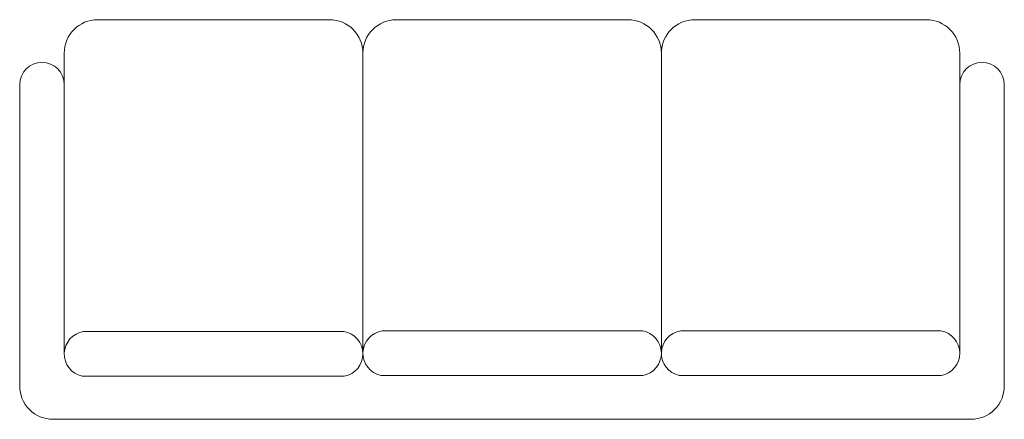
# Model space of a CAD drawing. Units: inches. Extents: x 94 to 277359, y -289541 to 1081.
# Tile 1 of 5: x 276565 to 277359, y -289541 to -289219. Entities that reach past the tile are written whole.
import ezdxf

# ---------------------------------------------------------------- set-up
doc = ezdxf.new("R2010")
doc.units = ezdxf.units.IN
doc.header["$MEASUREMENT"] = 0
doc.layers.add('FURN', color=150, linetype='Continuous', lineweight=5)
doc.layers.add('furniture', color=163, linetype='Continuous', lineweight=18)

# ---------------------------------------------------------------- blocks, each defined once
blk = doc.blocks.new('DOUBLE SOFA1')
at = {"layer": 'FURN'}
for p, q in [((23083.121, -24119.146), (23067.573, -24119.146)), ((23067.573, -24119.146), (23067.573, -24119.146)), ((23083.121, -24119.146), (23083.121, -24119.146)), ((23087.629, -24119.146), (23103.177, -24119.146)), ((23103.156, -24119.146), (23103.156, -24119.146)), ((23107.664, -24119.146), (23123.213, -24119.146)), ((23123.192, -24119.146), (23123.192, -24119.146)), ((23085.385, -24141.558), (23085.385, -24121.39)), ((23105.421, -24141.558), (23105.421, -24121.39))]:
    blk.add_line(p, q, dxfattribs=at)
for points in [[(23065.33, -24141.662), (23065.33, -24121.39)], [(23105.421, -24141.57), (23105.421, -24121.39)], [(23125.456, -24141.57), (23125.456, -24121.39)], [(23084.113, -24140.1), (23066.628, -24140.1)], [(23104.149, -24140.053), (23086.685, -24140.053)], [(23124.184, -24140.053), (23106.72, -24140.053)]]:
    blk.add_lwpolyline(points, dxfattribs=at)
for points in [[(23065.33, -24123.514, 0.999447), (23062.338, -24123.514), (23062.338, -24123.514), (23062.338, -24143.746), (23062.338, -24143.746, 0.414214), (23064.582, -24145.99), (23064.582, -24145.99), (23126.204, -24145.989), (23126.204, -24145.989, 0.414214), (23128.448, -24143.746), (23128.448, -24143.746), (23128.448, -24123.513), (23128.448, -24123.513, 1), (23125.456, -24123.515)], [(23066.628, -24140.1, 0.834492), (23066.527, -24143.091, 0.834492)], [(23084.113, -24140.1, -0.843667), (23084.133, -24143.091), (23084.133, -24143.091), (23066.527, -24143.091)], [(23086.685, -24140.053, 0.834492), (23086.583, -24143.044)], [(23104.149, -24140.053, -0.843667), (23104.169, -24143.044), (23104.169, -24143.044), (23086.583, -24143.044)], [(23106.72, -24140.053, 0.834492), (23106.619, -24143.044)], [(23124.184, -24140.053, -0.843667), (23124.204, -24143.044), (23124.204, -24143.044), (23106.619, -24143.044)]]:
    blk.add_lwpolyline(points, format="xyb", dxfattribs=at)
for centre, start, end in [((23067.573, -24121.39), 90, 180), ((23083.141, -24121.39), 0, 90), ((23087.629, -24121.39), 90, 180), ((23103.177, -24121.39), 0, 90), ((23103.177, -24121.39), 0, 90), ((23107.664, -24121.39), 90, 180), ((23123.213, -24121.39), 0, 90), ((23123.213, -24121.39), 0, 90)]:
    blk.add_arc(centre, 2.244, start, end, dxfattribs=at)

msp = doc.modelspace()

# ---------------------------------------------------------------- block references
at = {"layer": 'furniture', "xscale": 12, "yscale": 12, "zscale": 12}
msp.add_blockref('DOUBLE SOFA1', (-182.81, 211.18), dxfattribs=at)

doc.saveas('drawing.dxf')
